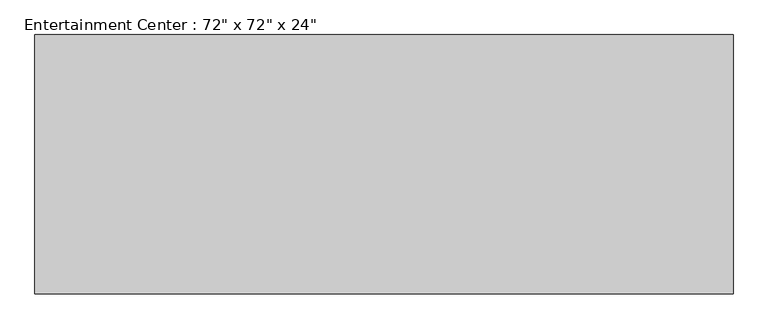
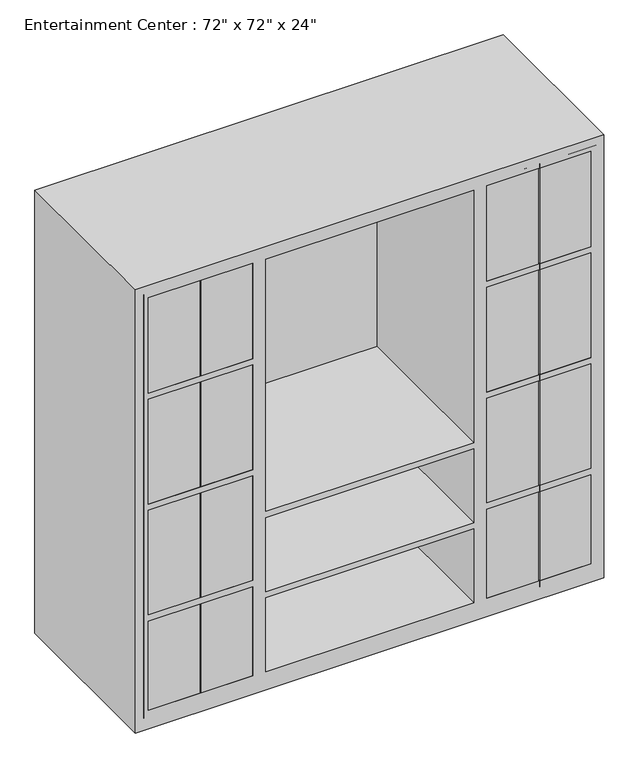
"""IFC4 building model written with IfcOpenShell, lengths in millimetres: furniture geometry."""

from ifc_helpers import new_model, si_unit, point, frame, frame_2d, origin, place, context, project, spatial, polyline, circle_curve, trimmed, segment, composite_curve, outline, extrude, faceted_brep, source, transform, mapped, element, save


def furniture_cf0b6580(model_context):
    return source(origin(), model_context, "Body", "SolidModel", [
        faceted_brep([(914.4, -781.05, 0.0), (914.4, -781.05, 1828.8), (-914.4, -781.05, 1828.8), (-914.4, -781.05, 0.0), (-457.2, -781.05, 1778.0), (-457.2, -781.05, 1384.3), (-863.6, -781.05, 1384.3), (-863.6, -781.05, 1778.0), (-457.2, -781.05, 76.2), (-863.6, -781.05, 76.2), (-863.6, -781.05, 444.5), (-457.2, -781.05, 444.5), (863.6, -781.05, 1384.3), (457.2, -781.05, 1384.3), (457.2, -781.05, 1778.0), (863.6, -781.05, 1778.0), (-406.4, -781.05, 736.6), (-406.4, -781.05, 1778.0), (406.4, -781.05, 1778.0), (406.4, -781.05, 736.6), (406.4, -781.05, 76.2), (-406.4, -781.05, 76.2), (-406.4, -781.05, 381.0), (406.4, -781.05, 381.0), (863.6, -781.05, 76.2), (457.2, -781.05, 76.2), (457.2, -781.05, 444.5), (863.6, -781.05, 444.5), (-863.6, -781.05, 469.9), (-863.6, -781.05, 901.7), (-457.2, -781.05, 901.7), (-457.2, -781.05, 469.9), (-457.2, -781.05, 1358.9), (-457.2, -781.05, 927.1), (-863.6, -781.05, 927.1), (-863.6, -781.05, 1358.9), (457.2, -781.05, 1358.9), (863.6, -781.05, 1358.9), (863.6, -781.05, 927.1), (457.2, -781.05, 927.1), (457.2, -781.05, 901.7), (863.6, -781.05, 901.7), (863.6, -781.05, 469.9), (457.2, -781.05, 469.9), (406.4, -781.05, 406.4), (-406.4, -781.05, 406.4), (-406.4, -781.05, 711.2), (406.4, -781.05, 711.2), (914.4, -101.6, 0.0), (-914.4, -101.6, 0.0), (-914.4, -101.6, 1828.8), (914.4, -101.6, 1828.8), (-457.2, -127.0, 1778.0), (-457.2, -127.0, 1384.3), (-863.6, -127.0, 1384.3), (-863.6, -127.0, 1778.0), (-457.2, -127.0, 76.2), (-863.6, -127.0, 76.2), (-863.6, -127.0, 444.5), (-457.2, -127.0, 444.5), (863.6, -127.0, 1384.3), (457.2, -127.0, 1384.3), (457.2, -127.0, 1778.0), (863.6, -127.0, 1778.0), (-406.4, -127.0, 736.6), (-406.4, -127.0, 1778.0), (406.4, -127.0, 1778.0), (406.4, -127.0, 736.6), (406.4, -127.0, 76.2), (-406.4, -127.0, 76.2), (-406.4, -127.0, 381.0), (406.4, -127.0, 381.0), (863.6, -127.0, 76.2), (457.2, -127.0, 76.2), (457.2, -127.0, 444.5), (863.6, -127.0, 444.5), (-863.6, -127.0, 469.9), (-863.6, -127.0, 901.7), (-457.2, -127.0, 901.7), (-457.2, -127.0, 469.9), (-457.2, -127.0, 1358.9), (-457.2, -127.0, 927.1), (-863.6, -127.0, 927.1), (-863.6, -127.0, 1358.9), (457.2, -127.0, 1358.9), (863.6, -127.0, 1358.9), (863.6, -127.0, 927.1), (457.2, -127.0, 927.1), (457.2, -127.0, 901.7), (863.6, -127.0, 901.7), (863.6, -127.0, 469.9), (457.2, -127.0, 469.9), (406.4, -127.0, 406.4), (-406.4, -127.0, 406.4), (-406.4, -127.0, 711.2), (406.4, -127.0, 711.2)], [[[0, 1, 2, 3], [4, 5, 6, 7], [8, 9, 10, 11], [12, 13, 14, 15], [16, 17, 18, 19], [20, 21, 22, 23], [24, 25, 26, 27], [28, 29, 30, 31], [32, 33, 34, 35], [36, 37, 38, 39], [40, 41, 42, 43], [44, 45, 46, 47]], [[48, 49, 50, 51]], [[1, 0, 48, 51]], [[2, 1, 51, 50]], [[3, 2, 50, 49]], [[0, 3, 49, 48]], [[5, 4, 52, 53]], [[6, 5, 53, 54]], [[7, 6, 54, 55]], [[4, 7, 55, 52]], [[9, 8, 56, 57]], [[10, 9, 57, 58]], [[11, 10, 58, 59]], [[8, 11, 59, 56]], [[13, 12, 60, 61]], [[14, 13, 61, 62]], [[15, 14, 62, 63]], [[12, 15, 63, 60]], [[17, 16, 64, 65]], [[18, 17, 65, 66]], [[19, 18, 66, 67]], [[16, 19, 67, 64]], [[21, 20, 68, 69]], [[22, 21, 69, 70]], [[23, 22, 70, 71]], [[20, 23, 71, 68]], [[25, 24, 72, 73]], [[26, 25, 73, 74]], [[27, 26, 74, 75]], [[24, 27, 75, 72]], [[29, 28, 76, 77]], [[30, 29, 77, 78]], [[31, 30, 78, 79]], [[28, 31, 79, 76]], [[33, 32, 80, 81]], [[34, 33, 81, 82]], [[35, 34, 82, 83]], [[32, 35, 83, 80]], [[37, 36, 84, 85]], [[38, 37, 85, 86]], [[39, 38, 86, 87]], [[36, 39, 87, 84]], [[41, 40, 88, 89]], [[42, 41, 89, 90]], [[43, 42, 90, 91]], [[40, 43, 91, 88]], [[45, 44, 92, 93]], [[46, 45, 93, 94]], [[47, 46, 94, 95]], [[44, 47, 95, 92]], [[53, 52, 55, 54]], [[57, 56, 59, 58]], [[61, 60, 63, 62]], [[65, 64, 67, 66]], [[69, 68, 71, 70]], [[73, 72, 75, 74]], [[77, 76, 79, 78]], [[81, 80, 83, 82]], [[85, 84, 87, 86]], [[89, 88, 91, 90]], [[93, 92, 95, 94]]]),
        extrude(outline(composite_curve([segment(polyline([(1003.3, -632.9986452), (1003.3, -657.225), (825.5, -657.225), (825.5, -632.9986452)]), True, "CONTINUOUS"), segment(trimmed(circle_curve(frame_2d((850.9, -632.9986452)), 25.4), [point((825.5, -632.9986452))], [point((850.9, -607.5986452))], False, "CARTESIAN"), True, "CONTINUOUS"), segment(polyline([(850.9, -607.5986452), (977.9, -607.5986452)]), True, "CONTINUOUS"), segment(trimmed(circle_curve(frame_2d((977.9, -632.9986452)), 25.4), [point((977.9, -607.5986452))], [point((1003.3, -632.9986452))], False, "CARTESIAN"), True, "CONTINUOUS")], self_intersect=False)), frame((0.0, -714.375, 0.0), z_axis=(0.0, 1.0, 0.0), x_axis=(0.0, 0.0, 1.0)), (0.0, 0.0, 1.0), 3.175),
        extrude(outline(composite_curve([segment(trimmed(circle_curve(frame_2d((977.9, -688.18125)), 25.4), [point((1003.3, -688.18125))], [point((977.9, -713.58125))], False, "CARTESIAN"), True, "CONTINUOUS"), segment(polyline([(977.9, -713.58125), (850.9, -713.58125)]), True, "CONTINUOUS"), segment(trimmed(circle_curve(frame_2d((850.9, -688.18125)), 25.4), [point((850.9, -713.58125))], [point((825.5, -688.18125))], False, "CARTESIAN"), True, "CONTINUOUS"), segment(polyline([(825.5, -688.18125), (825.5, -663.575), (1003.3, -663.575), (1003.3, -688.18125)]), True, "CONTINUOUS")], self_intersect=False)), frame((0.0, -714.375, 0.0), z_axis=(0.0, 1.0, 0.0), x_axis=(0.0, 0.0, 1.0)), (0.0, 0.0, 1.0), 3.175),
        extrude(outline(composite_curve([segment(trimmed(circle_curve(frame_2d((977.9, 632.9986452)), 25.4), [point((1003.3, 632.9986452))], [point((977.9, 607.5986452))], False, "CARTESIAN"), True, "CONTINUOUS"), segment(polyline([(977.9, 607.5986452), (850.9, 607.5986452)]), True, "CONTINUOUS"), segment(trimmed(circle_curve(frame_2d((850.9, 632.9986452)), 25.4), [point((850.9, 607.5986452))], [point((825.5, 632.9986452))], False, "CARTESIAN"), True, "CONTINUOUS"), segment(polyline([(825.5, 632.9986452), (825.5, 657.225), (1003.3, 657.225), (1003.3, 632.9986452)]), True, "CONTINUOUS")], self_intersect=False)), frame((0.0, -714.375, 0.0), z_axis=(0.0, 1.0, 0.0), x_axis=(0.0, 0.0, 1.0)), (0.0, 0.0, 1.0), 3.175),
        extrude(outline(composite_curve([segment(polyline([(1003.3, 688.18125), (1003.3, 663.575), (825.5, 663.575), (825.5, 688.18125)]), True, "CONTINUOUS"), segment(trimmed(circle_curve(frame_2d((850.9, 688.18125)), 25.4), [point((825.5, 688.18125))], [point((850.9, 713.58125))], False, "CARTESIAN"), True, "CONTINUOUS"), segment(polyline([(850.9, 713.58125), (977.9, 713.58125)]), True, "CONTINUOUS"), segment(trimmed(circle_curve(frame_2d((977.9, 688.18125)), 25.4), [point((977.9, 713.58125))], [point((1003.3, 688.18125))], False, "CARTESIAN"), True, "CONTINUOUS")], self_intersect=False)), frame((0.0, -714.375, 0.0), z_axis=(0.0, 1.0, 0.0), x_axis=(0.0, 0.0, 1.0)), (0.0, 0.0, 1.0), 3.175),
        extrude(outline(polyline([(-882.65, -711.2), (-663.575, -711.2), (-663.575, -781.05), (-882.65, -781.05), (-882.65, -711.2)])), frame((0.0, 0.0, 50.8), z_axis=(0.0, 0.0, 1.0), x_axis=(1.0, 0.0, 0.0)), (0.0, 0.0, 1.0), 1746.25),
        extrude(outline(polyline([(-657.225, -711.2), (-438.15, -711.2), (-438.15, -781.05), (-657.225, -781.05), (-657.225, -711.2)])), frame((0.0, 0.0, 50.8), z_axis=(0.0, 0.0, 1.0), x_axis=(1.0, 0.0, 0.0)), (0.0, 0.0, 1.0), 1746.25),
        extrude(outline(polyline([(663.575, -711.2), (882.65, -711.2), (882.65, -781.05), (663.575, -781.05), (663.575, -711.2)])), frame((0.0, 0.0, 50.8), z_axis=(0.0, 0.0, 1.0), x_axis=(1.0, 0.0, 0.0)), (0.0, 0.0, 1.0), 1746.25),
        extrude(outline(polyline([(438.15, -711.2), (657.225, -711.2), (657.225, -781.05), (438.15, -781.05), (438.15, -711.2)])), frame((0.0, 0.0, 50.8), z_axis=(0.0, 0.0, 1.0), x_axis=(1.0, 0.0, 0.0)), (0.0, 0.0, 1.0), 1746.25),
    ])


if __name__ == "__main__":
    model = new_model("IFC4")
    model_context = context("Model", 3, world=origin())
    ifc_project = project(units=[si_unit("LENGTHUNIT", "METRE", prefix="MILLI")], contexts=[model_context])
    site = spatial("IfcSite", under=ifc_project)
    building = spatial("IfcBuilding", under=site)
    placement = place(None, origin())
    furniture_shape = furniture_cf0b6580(model_context)
    element("IfcFurniture", 1, ObjectType="Entertainment Center : 72\" x 72\" x 24\"", at=placement, inside=building, context=model_context, shape_type="MappedRepresentation", body=[
        mapped(furniture_shape, transform((0.0, 0.0, 0.0), x_axis=(1.0, 0.0, 0.0), y_axis=(0.0, 1.0, 0.0), z_axis=(0.0, 0.0, 1.0))),
    ])
    save(model, "model.ifc")

# Revit data of these elements
# Type "Entertainment Center : 72\" x 72\" x 24\""
#   Assembly Code = "E2020200"
#   Center Width = 2' - 8"
#   Depth = 2' - 0"
#   Height = 6' - 0"
#   Width = 6' - 0"
#   Material = Wood - Teak
#   Default Elevation = 0
# Element 1 (IfcFurniture, "Entertainment Center : 72\" x 72\" x 24\"")
#   Materials on its faces: "Wood - Teak", "Steel, Chrome Plated", "Glass - Clear, Grey"
# Materials
#   "Wood - Teak": class "Wood", colour RGB 145 112 90, transparency 0
#   "Steel, Chrome Plated": class "Metal", colour RGB 17 17 17, transparency 0, Description = "Chromiuim plated steel", Cost = 0
#   "Glass - Clear, Grey": class "Glass", colour RGB 252 255 255, transparency 0.64
